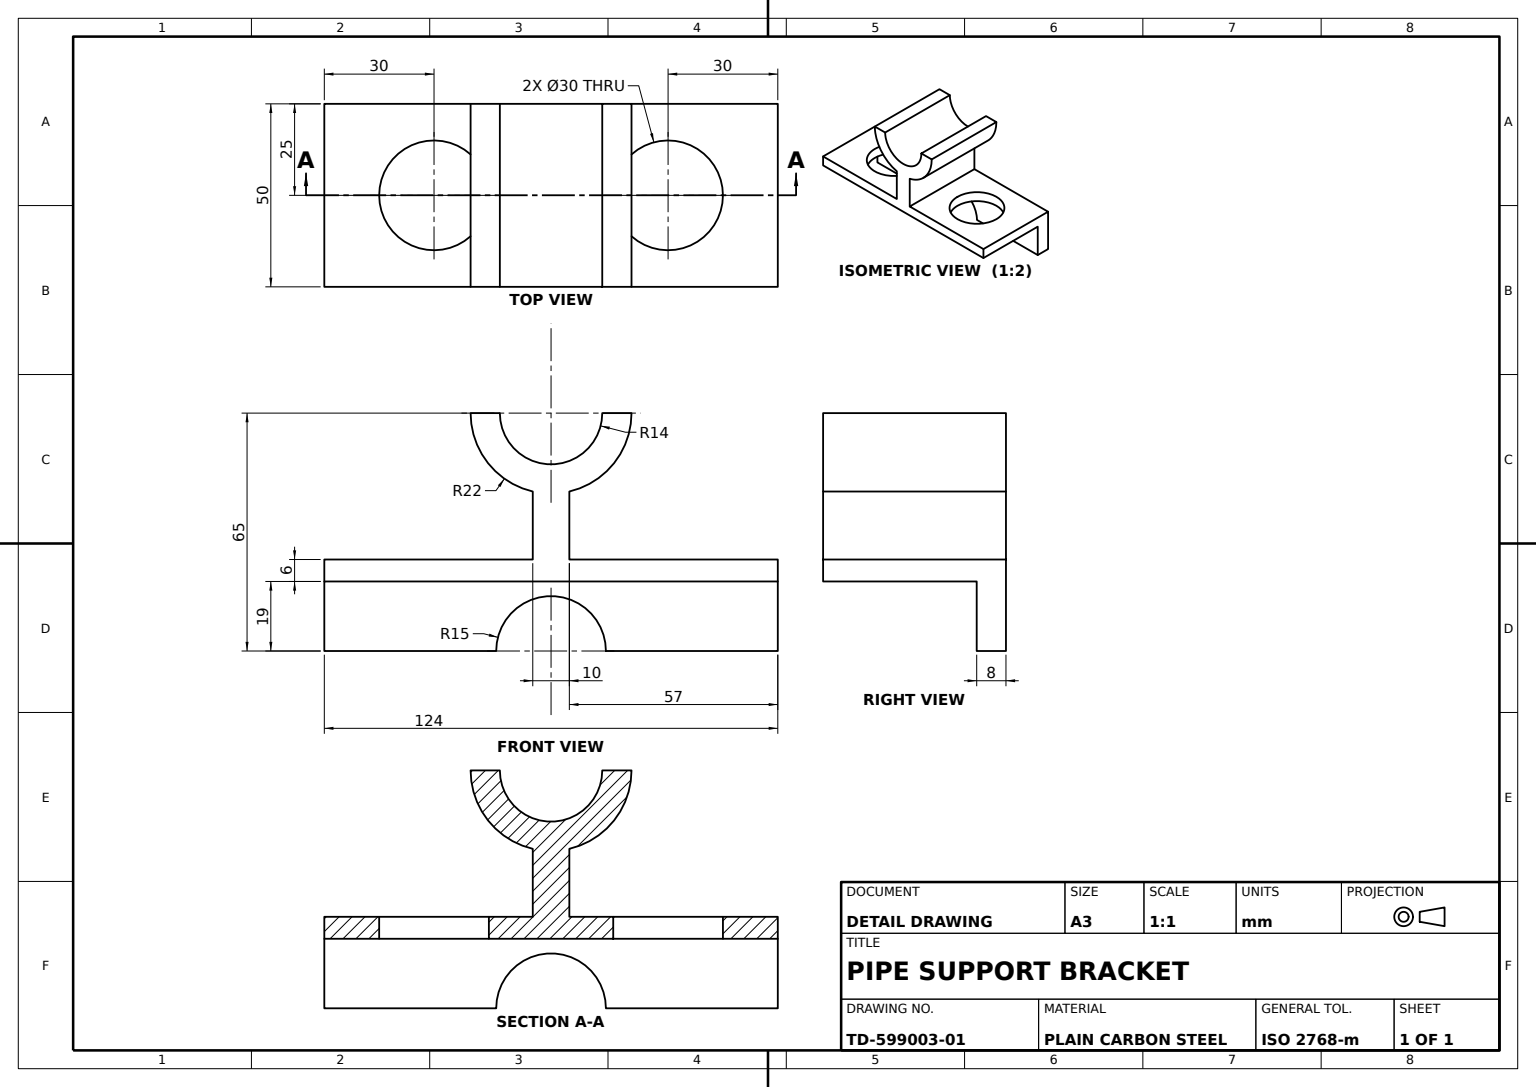
SolidWorks part; units mm, degrees
material "Plain Carbon Steel"
ref_plane "Front Plane" through (0, 0, 0) normal (0, 0, 1) x (1, 0, 0)
ref_plane "Top Plane" through (0, 0, 0) normal (0, 1, 0) x (1, 0, 0)
ref_plane "Right Plane" through (0, 0, 0) normal (1, 0, 0) x (0, 0, -1)
sketch "Base Angle Profile Sketch" plane through (0, 0, 0) normal (0, 0, 1) x (1, 0, 0)
  line L0 (0, 0) -> (0, 25)
  line L1 (0, 25) -> (50, 25)
  line L2 (0, 0) -> (8, 0)
  line L3 (50, 25) -> (50, 19)
  line L4 (50, 19) -> (8, 19)
  line L5 (8, 19) -> (8, 0)
  dimension "D1" = 50
  dimension "D2" = 42
  dimension "D3" = 25
  dimension "D4" = 6
  dimension "D5" = 8
extrude "Base Angle" add sketch "Base Angle Profile Sketch" along normal blind 124
sketch "Saddle Boss Sketch" plane through (0, 0, 0) normal (-1, 0, 0) x (0, 0, 1)
  line L1 (124, 25) -> (0, 25) construction
  line L4 (62, 65) -> (40, 65)
  line L5 (40, 65) -> (84, 65)
  line L6 (57, 25) -> (57, 43.5757)
  line L7 (67, 25) -> (67, 43.5757)
  line L8 (124, 0) -> (0, 0) construction
  arc A0 (67, 43.5757) -> (84, 65) centre (62, 65) ccw
  arc A1 (40, 65) -> (57, 43.5757) centre (62, 65) ccw
  line M4 (124, 25) -> (0, 25)
  dimension "D1" = 22
  dimension "D2" = 40
  dimension "D3" = 57
  dimension "D4" = 43.5757
extrude "Saddle Boss" add sketch "Saddle Boss Sketch" against normal blind 50 contours L4 A1 L6 L7 A0 L5 M4
sketch "Saddle Seat Sketch" plane through (0, 0, 0) normal (-1, 0, 0) x (0, 0, 1)
  line L0 (84, 65) -> (40, 65) construction
  line L1 (48, 65) -> (76, 65)
  arc A0 (48, 65) -> (76, 65) centre (62, 65) ccw
  dimension "D1" = 14
extrude "Saddle Seat Cut" cut sketch "Saddle Seat Sketch" against normal blind 50
sketch "Relief Cut Sketch" plane through (0, 0, 0) normal (-1, 0, 0) x (0, 0, 1)
  line L0 (124, 0) -> (0, 0) construction
  line L1 (47, 0) -> (77, 0)
  arc A0 (77, 0) -> (47, 0) centre (62, 0) ccw
  dimension "D1" = 15
extrude "Relief Cut" cut sketch "Relief Cut Sketch" against normal blind 50
sketch "Mounting Holes Sketch" plane through (0, 19, 0) normal (0, -1, 0) x (1, 0, 0)
  line L0 (0, 47) -> (0, 0) construction
  line L1 (8, 0) -> (50, 0) construction
  line L2 (0, 124) -> (0, 77) construction
  line L3 (8, 124) -> (50, 124) construction
  circle A0 centre (25, 94) radius 15
  circle A1 centre (25, 30) radius 15
  dimension "D1" = 25
  dimension "D5" = 30
  dimension "D2" = 30
  dimension "D3" = 25
  dimension "D4" = 30
extrude "Mounting Holes 2xØ30" cut sketch "Mounting Holes Sketch" against normal blind 20
